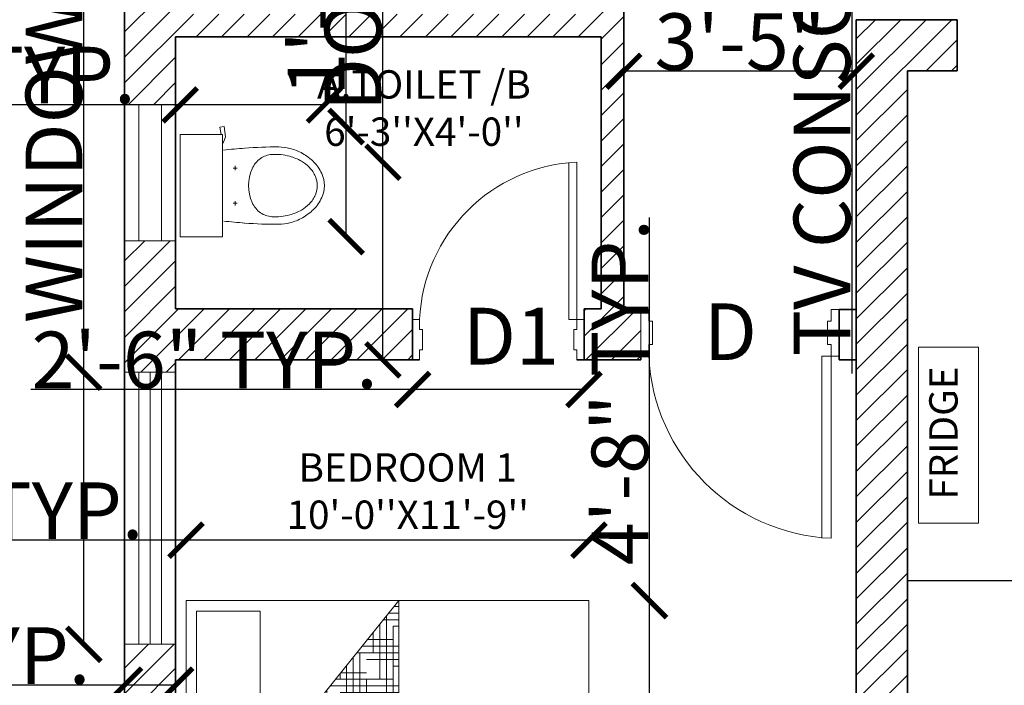
# Model space of a CAD drawing. Units: inches. Extents: x 1957 to 2456, y 1504 to 2088.
# Tile 3 of 6: x 2047 to 2220, y 1703 to 1820. Entities that reach past the tile are written whole.
import ezdxf

# ---------------------------------------------------------------- set-up
doc = ezdxf.new("R2010")
doc.units = ezdxf.units.IN
doc.header["$LTSCALE"] = 2
for name, color, linetype, lineweight in [('A-ANNO-DIMS', 2, 'Continuous', 18), ('A-ANNO-TEXT', 7, 'Continuous', 18), ('A-AREA-IDEN', 7, 'Continuous', 18), ('A-EQPM', 8, 'Continuous', 18), ('A-FLOR-FIXT', 8, 'Continuous', 18), ('A-FURN', 8, 'Continuous', 18), ('A-WALL-PATT', 8, 'Continuous', 13), ('Doors', 42, 'Continuous', 18), ('Kitchen', 60, 'Continuous', 25), ('Walls', 7, 'Continuous', 35), ('Windows', 140, 'Continuous', 18)]:
    doc.layers.add(name, color=color, linetype=linetype, lineweight=lineweight)
doc.styles.get("Standard").update_dxf_attribs({"font": 'arial.ttf'})
doc.dimstyles.get("Standard").update_dxf_attribs({"dimtxt": 10, "dimasz": 6, "dimexe": 0.18, "dimexo": 0.0625, "dimgap": 0.09, "dimtad": 1, "dimdec": 1, "dimzin": 0, "dimdsep": 46, "dimlunit": 4, "dimtxsty": 'Standard', "dimblk": 'ARCHTICK', "dimcen": 0.09, "dimse1": 1, "dimse2": 1, "dimadec": 0, "dimazin": 0, "dimtfac": 1, "dimtdec": 1, "dimtofl": 0, "dimtmove": 0, "dimatfit": 3, "dimfxl": 1, "dimtolj": 1, "dimtzin": 0, "dimarcsym": 0})

# ---------------------------------------------------------------- blocks, each defined once
blk = doc.blocks.new('*X4')
at = {"color": 0}
for p, q in [((20.25, 14.8125), (20.2772, 14.8125)), ((20.1875, 14.75), (20.1875, 14.7669)), ((20.199, 14.7812), (20.2772, 14.7812)), ((20.1487, 14.7188), (20.2772, 14.7188)), ((20.1562, 14.625), (20.1562, 14.7281)), ((20.1739, 14.75), (20.2772, 14.75)), ((20.25, 14.3194), (20.25, 14.75)), ((20.1236, 14.6875), (20.25, 14.6875)), ((20.125, 14.5), (20.125, 14.6893)), ((20.0938, 14.375), (20.0938, 14.6504)), ((20.0984, 14.6562), (20.125, 14.6562)), ((20.2188, 14.3091), (20.2188, 14.625)), ((20.25, 14.625), (20.2772, 14.625)), ((20.0625, 14.2573), (20.0625, 14.6116)), ((20.125, 14.5938), (20.2772, 14.5938)), ((19.9979, 14.5312), (20.2772, 14.5312)), ((20.023, 14.5625), (20.2772, 14.5625)), ((20.0312, 14.2469), (20.0312, 14.5727)), ((19.9727, 14.5), (20.25, 14.5)), ((20, 14.2366), (20, 14.5)), ((20.1875, 14.2987), (20.1875, 14.5)), ((19.9476, 14.4688), (20.125, 14.4688)), ((19.9062, 14.375), (19.9062, 14.4174)), ((19.9225, 14.4375), (20, 14.4375)), ((20.125, 14.4062), (20.2772, 14.4062)), ((20.25, 14.4375), (20.2772, 14.4375)), ((19.875, 14.25), (19.875, 14.3785)), ((19.9688, 14.2262), (19.9688, 14.375)), ((20, 14.375), (20.2772, 14.375)), ((20.1562, 14.2884), (20.1562, 14.375)), ((19.8125, 14.1744), (19.8125, 14.3008)), ((19.8219, 14.3125), (20.2291, 14.3125)), ((19.8438, 14.1848), (19.8438, 14.3397)), ((19.875, 14.3438), (20.2772, 14.3438)), ((19.7812, 14.1641), (19.7812, 14.262)), ((19.7967, 14.2812), (20.125, 14.2812)), ((19.7465, 14.2188), (19.875, 14.2188)), ((19.75, 14.1537), (19.75, 14.2231)), ((19.7716, 14.25), (20, 14.25)), ((19.9375, 14.2159), (19.9375, 14.25)), ((19.7213, 14.1875), (19.75, 14.1875)), ((19.7188, 14.0726), (19.7188, 14.1136)), ((19.7018, 14.0938), (19.7786, 14.0938)), ((19.75, 14.0338), (19.75, 14.1032)), ((19.7812, 13.9949), (19.7812, 14.0929)), ((19.8125, 14), (19.8125, 14.0825)), ((19.7269, 14.0625), (19.8728, 14.0625)), ((19.752, 14.0312), (19.875, 14.0312)), ((19.9062, 13.8396), (19.9062, 14.0514)), ((19.9375, 13.8007), (19.9375, 14.0411)), ((19.9688, 13.875), (19.9688, 14.0307)), ((19.875, 13.8784), (19.875, 14)), ((20, 14), (20, 14.0204)), ((20, 14), (20.0614, 14)), ((20.0625, 13.6454), (20.0625, 13.9996)), ((20.0938, 13.625), (20.0938, 13.9893)), ((20.125, 13.75), (20.125, 13.9789)), ((19.8275, 13.9375), (20.25, 13.9375)), ((19.875, 13.9688), (20.1557, 13.9688)), ((20.1562, 13.875), (20.1562, 13.9686)), ((20.25, 13.5), (20.25, 13.9375)), ((19.8526, 13.9062), (20.125, 13.9062)), ((19.8777, 13.875), (20, 13.875)), ((20.0312, 13.6842), (20.0312, 13.875)), ((20.125, 13.8438), (20.2772, 13.8438)), ((20.2188, 13.4511), (20.2188, 13.875)), ((20.25, 13.875), (20.2772, 13.875)), ((20, 13.8125), (20.2772, 13.8125)), ((19.9532, 13.7812), (20.2772, 13.7812)), ((19.9783, 13.75), (20.25, 13.75)), ((20, 13.723), (20, 13.75)), ((20.1875, 13.49), (20.1875, 13.75)), ((20.0035, 13.7188), (20.125, 13.7188)), ((20.125, 13.6562), (20.2772, 13.6562)), ((20.25, 13.6875), (20.2772, 13.6875)), ((20.0789, 13.625), (20.2772, 13.625)), ((20.1562, 13.5288), (20.1562, 13.625)), ((20.104, 13.5938), (20.2772, 13.5938)), ((20.1292, 13.5625), (20.25, 13.5625)), ((20.2046, 13.4688), (20.2772, 13.4688)), ((20.25, 13.5), (20.2772, 13.5)), ((20.2297, 13.4375), (20.2772, 13.4375)), ((20.2549, 13.4062), (20.2772, 13.4062))]:
    blk.add_line(p, q, dxfattribs=at)
blk = doc.blocks.new('MAT-P13')
for p, q in [((-0.75, 0), (0.75, 0)), ((-0.75, 0), (-0.75, -1.9)), ((0.75, 0), (0.75, -1.9)), ((-0.7, -0.05), (-0.7, -0.35)), ((-0.7, -0.05), (-0.05, -0.05)), ((-0.05, -0.35), (-0.05, -0.05)), ((0.05, -0.05), (0.7, -0.05)), ((0.05, -0.35), (0.05, -0.05)), ((0.7, -0.05), (0.7, -0.35)), ((-0.7, -0.35), (-0.05, -0.35)), ((0.05, -0.35), (0.7, -0.35)), ((-0.75, -1.0034), (0, -0.4)), ((0, -0.4), (-0.75, -1.0034)), ((0, -0.4), (-0.2, -1.0034)), ((0, -0.4), (0.2, -1.0034)), ((0, -0.4), (0.75, -1.0034)), ((-0.75, -1.0034), (-0.2, -1.0034)), ((0.2, -1.0034), (0.75, -1.0034)), ((0.75, -1.9), (-0.75, -1.9))]:
    blk.add_line(p, q)
at = {"xscale": -1, "rotation": 90}
blk.add_blockref('*X4', (14.1285, 19.2738), dxfattribs=at)
blk = doc.blocks.new('AP0B05')
for p, q in [((35, 100), (35, 880)), ((75, 100), (75, 878.9))]:
    blk.add_line(p, q)
for points in [[(0, 100), (0, -100), (35, -100), (35, -50), (50, -50), (50, 50), (35, 50), (35, 100)], [(850, 100), (850, -100), (815, -100), (815, -50), (800, -50), (800, 50), (815, 50), (815, 100)]]:
    blk.add_lwpolyline(points, close=True)
blk.add_lwpolyline([(35, 100), (75, 100)])
blk.add_arc((-2.4, 62.6), 818.3, 2.6212, 87.3788)
blk = doc.blocks.new('_ArchTick')
at = {"color": 0, "linetype": 'ByBlock', "const_width": 0.15}
blk.add_lwpolyline([(-0.5, -0.5), (0.5, 0.5)], dxfattribs=at)
blk = doc.blocks.new('*D10')
at = {"layer": 'A-ANNO-DIMS', "color": 0, "lineweight": -2, "transparency": 16777216}
blk.add_line((2194.03, 1811.13), (2153.03, 1811.13), dxfattribs=at)
at = {"layer": 'Defpoints', "color": 0, "transparency": 16777216}
for p in [(2153.03, 1820.22), (2194.03, 1820.22), (2153.03, 1811.13)]:
    blk.add_point(p, dxfattribs=at)
at = {"layer": 'A-ANNO-DIMS', "color": 0, "lineweight": -2, "transparency": 16777216, "xscale": 6, "yscale": 6, "zscale": 6, "rotation": 180}
blk.add_blockref('_ArchTick', (2153.03, 1811.13), dxfattribs=at)
at = {"layer": 'A-ANNO-DIMS', "color": 0, "lineweight": -2, "transparency": 16777216, "xscale": 6, "yscale": 6, "zscale": 6}
blk.add_blockref('_ArchTick', (2194.03, 1811.13), dxfattribs=at)
at = {"layer": 'A-ANNO-DIMS', "color": 0, "transparency": 16777216, "insert": (2173.53, 1816.33), "char_height": 10, "attachment_point": 5}
blk.add_mtext('\\A1;3\'-5"', dxfattribs=at)
blk = doc.blocks.new('toilet-1')
at = {"color": 0, "linetype": 'ByBlock'}
for p, q in [((-0.23, -0.02), (-0.23, -0.2116)), ((0.23, -0.02), (-0.23, -0.02)), ((0.23, -0.02), (0.23, -0.2116)), ((-0.23, -0.2116), (0.23, -0.2116)), ((0.1917, -0.2144), (0.2206, -0.225)), ((0.2206, -0.225), (0.266, -0.2187)), ((0.2633, -0.1997), (0.23, -0.2044)), ((0.266, -0.2187), (0.2633, -0.1997)), ((-0.0793, -0.2587), (-0.0793, -0.2778)), ((0.0794, -0.2587), (0.0794, -0.2778)), ((-0.0889, -0.2683), (-0.0697, -0.2683)), ((0.0889, -0.2683), (0.0698, -0.2683)), ((0, -0.6382), (0, -0.6382))]:
    blk.add_line(p, q, dxfattribs=at)
for centre, radius, start, end in [((3.5272, -0.6239), 3.7093, 173.6925, 175.1593), ((-3.527, -0.624), 3.7093, 4.8413, 6.3171), ((1.7368, -0.4519), 1.9109, 175.7698, 180.3758), ((-0.0312, -0.4465), 0.1114, 113.8997, 145.1485), ((0, -0.5169), 0.1884, 66.0939, 113.9061), ((0.0312, -0.4465), 0.1114, 34.8515, 66.1003), ((-1.7366, -0.4519), 1.9109, 359.6242, 4.2302), ((-0.0408, -0.4398), 0.0996, 145.1497, 175.881), ((0.0409, -0.4398), 0.0996, 4.119, 34.8503), ((0.0981, -0.4497), 0.2389, 175.8862, 195.5931), ((-0.098, -0.4497), 0.2389, 344.4069, 4.1138), ((0.0353, -0.463), 0.2093, 180.3747, 194.3375), ((-0.0351, -0.463), 0.2093, 345.6614, 359.6243), ((0.055, -0.458), 0.2297, 194.3353, 209.622), ((0.0961, -0.4503), 0.2369, 195.5969, 209.3771), ((-0.096, -0.4503), 0.2369, 330.6229, 344.4031), ((-0.0548, -0.458), 0.2297, 330.3788, 345.6655), ((0.0647, -0.4524), 0.2409, 209.6273, 224.5489), ((0.0232, -0.4913), 0.1532, 209.3871, 226.5438), ((-0.0231, -0.4913), 0.1532, 313.4562, 330.6129), ((-0.0645, -0.4524), 0.2409, 315.4504, 330.372), ((0.0152, -0.4997), 0.1416, 226.5501, 246.5527), ((-0.0151, -0.4997), 0.1416, 293.4473, 313.4499), ((0.0178, -0.4986), 0.1751, 224.552, 245.714), ((0.0004, -0.538), 0.132, 245.5845, 269.8782), ((0, -0.5347), 0.1034, 246.5493, 270.0042), ((0, -0.5347), 0.1034, 269.9958, 293.4507), ((-0.0002, -0.538), 0.132, 270.1216, 294.4153), ((-0.0176, -0.4986), 0.1751, 294.2865, 315.4485)]:
    blk.add_arc(centre, radius, start, end, dxfattribs=at)
blk = doc.blocks.new('WIN-48IN')
for p, q in [((0, 6.5), (48, 6.5)), ((0, 4.5), (48, 4.5)), ((0, 2.5), (48, 2.5))]:
    blk.add_line(p, q)
blk.add_lwpolyline([(0, 9), (48, 9), (48, 0), (0, 0)], close=True)
blk = doc.blocks.new('VENT-WIN-24IN')
for p, q in [((2.5, 0), (2.5, 24)), ((6.5, 0), (6.5, 24))]:
    blk.add_line(p, q)
blk.add_lwpolyline([(0, 0), (0, 24), (9, 24), (9, 0)], close=True)
blk = doc.blocks.new('*D21')
at = {"layer": 'A-ANNO-DIMS', "color": 0, "lineweight": -2, "transparency": 16777216}
for p, q in [((2110.57, 1795.08), (2110.57, 1937.02)), ((2110.57, 1760.22), (2110.57, 1795.08))]:
    blk.add_line(p, q, dxfattribs=at)
at = {"layer": 'Defpoints', "color": 0, "transparency": 16777216}
for p in [(2110.57, 1795.08), (2115.8, 1795.08), (2115.8, 1760.22)]:
    blk.add_point(p, dxfattribs=at)
at = {"layer": 'A-ANNO-DIMS', "color": 0, "lineweight": -2, "transparency": 16777216, "xscale": 6, "yscale": 6, "zscale": 6}
for p, rotation in [((2110.57, 1795.08), 90), ((2110.57, 1760.22), 270)]:
    blk.add_blockref('_ArchTick', p, dxfattribs=dict(at, rotation=rotation))
at = {"layer": 'A-ANNO-DIMS', "color": 0, "transparency": 16777216, "insert": (2105.3, 1869.05), "char_height": 10, "attachment_point": 5, "rotation": 90}
blk.add_mtext('\\A1;DOOR D1 2\'-11" TYP.', dxfattribs=at)
blk = doc.blocks.new('*D22')
at = {"layer": 'A-ANNO-DIMS', "color": 0, "lineweight": -2, "transparency": 16777216}
for p, q in [((2115.8, 1754.99), (2048.49, 1754.99)), ((2146.03, 1754.99), (2115.8, 1754.99))]:
    blk.add_line(p, q, dxfattribs=at)
at = {"layer": 'Defpoints', "color": 0, "transparency": 16777216}
for p in [(2115.8, 1760.22), (2146.03, 1760.22), (2115.8, 1754.99)]:
    blk.add_point(p, dxfattribs=at)
at = {"layer": 'A-ANNO-DIMS', "color": 0, "lineweight": -2, "transparency": 16777216, "xscale": 6, "yscale": 6, "zscale": 6, "rotation": 180}
blk.add_blockref('_ArchTick', (2115.8, 1754.99), dxfattribs=at)
at = {"layer": 'A-ANNO-DIMS', "color": 0, "lineweight": -2, "transparency": 16777216, "xscale": 6, "yscale": 6, "zscale": 6}
blk.add_blockref('_ArchTick', (2146.03, 1754.99), dxfattribs=at)
at = {"layer": 'A-ANNO-DIMS', "color": 0, "transparency": 16777216, "insert": (2079.14, 1760.19), "char_height": 10, "attachment_point": 5}
blk.add_mtext('\\A1;2\'-6" TYP.', dxfattribs=at)
blk = doc.blocks.new('*D23')
at = {"layer": 'A-ANNO-DIMS', "color": 0, "lineweight": -2, "transparency": 16777216}
for p, q in [((2057.83, 1758.05), (2057.83, 1890.77)), ((2057.83, 1710.05), (2057.83, 1758.05))]:
    blk.add_line(p, q, dxfattribs=at)
at = {"layer": 'Defpoints', "color": 0, "transparency": 16777216}
for p in [(2057.83, 1758.05), (2065.03, 1758.05), (2065.03, 1710.05)]:
    blk.add_point(p, dxfattribs=at)
at = {"layer": 'A-ANNO-DIMS', "color": 0, "lineweight": -2, "transparency": 16777216, "xscale": 6, "yscale": 6, "zscale": 6}
for p, rotation in [((2057.83, 1758.05), 90), ((2057.83, 1710.05), 270)]:
    blk.add_blockref('_ArchTick', p, dxfattribs=dict(at, rotation=rotation))
at = {"layer": 'A-ANNO-DIMS', "color": 0, "transparency": 16777216, "insert": (2052.57, 1827.41), "char_height": 10, "attachment_point": 5, "rotation": 90}
blk.add_mtext('\\A1;WINDOW 4\'-0" TYP.', dxfattribs=at)
blk = doc.blocks.new('*D24')
at = {"layer": 'A-ANNO-DIMS', "color": 0, "lineweight": -2, "transparency": 16777216}
for p, q in [((2065.03, 1702.85), (1997.9, 1702.85)), ((2074.03, 1702.85), (2065.03, 1702.85))]:
    blk.add_line(p, q, dxfattribs=at)
at = {"layer": 'Defpoints', "color": 0, "transparency": 16777216}
for p in [(2065.03, 1710.05), (2074.03, 1710.05), (2065.03, 1702.85)]:
    blk.add_point(p, dxfattribs=at)
at = {"layer": 'A-ANNO-DIMS', "color": 0, "lineweight": -2, "transparency": 16777216, "xscale": 6, "yscale": 6, "zscale": 6}
for p, rotation in [((2065.03, 1702.85), 179.9999999999986), ((2074.03, 1702.85), 359.9999999999986)]:
    blk.add_blockref('_ArchTick', p, dxfattribs=dict(at, rotation=rotation))
at = {"layer": 'A-ANNO-DIMS', "color": 0, "transparency": 16777216, "insert": (2028.47, 1708.05), "char_height": 10, "attachment_point": 5}
blk.add_mtext('\\A1;0\'-9" TYP.', dxfattribs=at)
blk = doc.blocks.new('*D28')
at = {"layer": 'A-ANNO-DIMS', "color": 0, "lineweight": -2, "transparency": 16777216}
for p, q in [((2065.03, 1829.62), (2074.03, 1829.62)), ((2074.03, 1829.62), (2141.17, 1829.62))]:
    blk.add_line(p, q, dxfattribs=at)
at = {"layer": 'Defpoints', "color": 0, "transparency": 16777216}
for p in [(2065.03, 1833.22), (2074.03, 1833.22), (2074.03, 1829.62)]:
    blk.add_point(p, dxfattribs=at)
at = {"layer": 'A-ANNO-DIMS', "color": 0, "lineweight": -2, "transparency": 16777216, "xscale": 6, "yscale": 6, "zscale": 6, "rotation": 180}
blk.add_blockref('_ArchTick', (2065.03, 1829.62), dxfattribs=at)
at = {"layer": 'A-ANNO-DIMS', "color": 0, "lineweight": -2, "transparency": 16777216, "xscale": 6, "yscale": 6, "zscale": 6}
blk.add_blockref('_ArchTick', (2074.03, 1829.62), dxfattribs=at)
at = {"layer": 'A-ANNO-DIMS', "color": 0, "transparency": 16777216, "insert": (2110.6, 1834.81), "char_height": 10, "attachment_point": 5}
blk.add_mtext('\\A1;0\'-9" TYP.', dxfattribs=at)
blk = doc.blocks.new('*D29')
at = {"layer": 'A-ANNO-DIMS', "color": 0, "lineweight": -2, "transparency": 16777216}
for p, q in [((2075.86, 1728.42), (1968.79, 1728.42)), ((2146.9, 1728.42), (2075.86, 1728.42))]:
    blk.add_line(p, q, dxfattribs=at)
at = {"layer": 'Defpoints', "color": 0, "transparency": 16777216}
for p in [(2075.86, 1728.42), (2075.86, 1717.76), (2146.9, 1717.76)]:
    blk.add_point(p, dxfattribs=at)
at = {"layer": 'A-ANNO-DIMS', "color": 0, "lineweight": -2, "transparency": 16777216, "xscale": 6, "yscale": 6, "zscale": 6, "rotation": 180}
blk.add_blockref('_ArchTick', (2075.86, 1728.42), dxfattribs=at)
at = {"layer": 'A-ANNO-DIMS', "color": 0, "lineweight": -2, "transparency": 16777216, "xscale": 6, "yscale": 6, "zscale": 6}
blk.add_blockref('_ArchTick', (2146.9, 1728.42), dxfattribs=at)
at = {"layer": 'A-ANNO-DIMS', "color": 0, "transparency": 16777216, "insert": (2019.32, 1733.61), "char_height": 10, "attachment_point": 5}
blk.add_mtext('\\A1;BED 5\'-11" TYP.', dxfattribs=at)
blk = doc.blocks.new('*D30')
at = {"layer": 'A-ANNO-DIMS', "color": 0, "lineweight": -2, "transparency": 16777216}
for p, q in [((2157.56, 1717.76), (2157.56, 1785.3)), ((2157.56, 1661.68), (2157.56, 1717.76))]:
    blk.add_line(p, q, dxfattribs=at)
at = {"layer": 'Defpoints', "color": 0, "transparency": 16777216}
for p in [(2146.9, 1717.76), (2157.56, 1717.76), (2146.9, 1661.68)]:
    blk.add_point(p, dxfattribs=at)
at = {"layer": 'A-ANNO-DIMS', "color": 0, "lineweight": -2, "transparency": 16777216, "xscale": 6, "yscale": 6, "zscale": 6}
for p, rotation in [((2157.56, 1717.76), 90), ((2157.56, 1661.68), 270)]:
    blk.add_blockref('_ArchTick', p, dxfattribs=dict(at, rotation=rotation))
at = {"layer": 'A-ANNO-DIMS', "color": 0, "transparency": 16777216, "insert": (2152.36, 1754.53), "char_height": 10, "attachment_point": 5, "rotation": 90}
blk.add_mtext('\\A1;4\'-8" TYP.', dxfattribs=at)
blk = doc.blocks.new('*D33')
at = {"layer": 'A-ANNO-DIMS', "color": 0, "lineweight": -2, "transparency": 16777216}
for p, q in [((2074.82, 1805.18), (1956.82, 1805.18)), ((2100.26, 1805.18), (2074.82, 1805.18))]:
    blk.add_line(p, q, dxfattribs=at)
at = {"layer": 'Defpoints', "color": 0, "transparency": 16777216}
for p in [(2074.82, 1805.18), (2074.82, 1801.36), (2100.26, 1801.36)]:
    blk.add_point(p, dxfattribs=at)
at = {"layer": 'A-ANNO-DIMS', "color": 0, "lineweight": -2, "transparency": 16777216, "xscale": 6, "yscale": 6, "zscale": 6, "rotation": 180}
blk.add_blockref('_ArchTick', (2074.82, 1805.18), dxfattribs=at)
at = {"layer": 'A-ANNO-DIMS', "color": 0, "lineweight": -2, "transparency": 16777216, "xscale": 6, "yscale": 6, "zscale": 6}
blk.add_blockref('_ArchTick', (2100.26, 1805.18), dxfattribs=at)
at = {"layer": 'A-ANNO-DIMS', "color": 0, "transparency": 16777216, "insert": (2012.82, 1810.44), "char_height": 10, "attachment_point": 5}
blk.add_mtext('\\A1;WC 2\'-1 1/2" TYP.', dxfattribs=at)
blk = doc.blocks.new('*D34')
at = {"layer": 'A-ANNO-DIMS', "color": 0, "lineweight": -2, "transparency": 16777216}
for p, q in [((2104.08, 1801.36), (2104.08, 1890.86)), ((2104.08, 1781.95), (2104.08, 1801.36))]:
    blk.add_line(p, q, dxfattribs=at)
at = {"layer": 'Defpoints', "color": 0, "transparency": 16777216}
for p in [(2100.26, 1801.36), (2104.08, 1801.36), (2100.26, 1781.95)]:
    blk.add_point(p, dxfattribs=at)
at = {"layer": 'A-ANNO-DIMS', "color": 0, "lineweight": -2, "transparency": 16777216, "xscale": 6, "yscale": 6, "zscale": 6}
for p, rotation in [((2104.08, 1801.36), 90), ((2104.08, 1781.95), 270)]:
    blk.add_blockref('_ArchTick', p, dxfattribs=dict(at, rotation=rotation))
at = {"layer": 'A-ANNO-DIMS', "color": 0, "transparency": 16777216, "insert": (2098.81, 1849.11), "char_height": 10, "attachment_point": 5, "rotation": 90}
blk.add_mtext('\\A1;1\'-7 1/2" TYP.', dxfattribs=at)
blk = doc.blocks.new('*D39')
at = {"layer": 'A-ANNO-DIMS', "color": 0, "lineweight": -2, "transparency": 16777216}
for p, q in [((2193.24, 1973.36), (2193.24, 1908.07)), ((2193.24, 1908.07), (2193.24, 1757.83))]:
    blk.add_line(p, q, dxfattribs=at)
at = {"layer": 'Defpoints', "color": 0, "transparency": 16777216}
for p in [(2203.03, 1973.36), (2193.24, 1908.07), (2203.03, 1908.07)]:
    blk.add_point(p, dxfattribs=at)
at = {"layer": 'A-ANNO-DIMS', "color": 0, "lineweight": -2, "transparency": 16777216, "xscale": 6, "yscale": 6, "zscale": 6}
for p, rotation in [((2193.24, 1973.36), 90), ((2193.24, 1908.07), 270)]:
    blk.add_blockref('_ArchTick', p, dxfattribs=dict(at, rotation=rotation))
at = {"layer": 'A-ANNO-DIMS', "color": 0, "transparency": 16777216, "insert": (2187.98, 1829.95), "char_height": 10, "attachment_point": 5, "rotation": 90}
blk.add_mtext('\\A1;TV CONSOLE 5\'-5 1/2"', dxfattribs=at)
blk = doc.blocks.new('*D52')
at = {"layer": 'A-ANNO-DIMS', "color": 0, "lineweight": -2, "transparency": 16777216}
blk.add_line((2040.63, 1610.22), (2040.63, 1710.05), dxfattribs=at)
at = {"layer": 'Defpoints', "color": 0, "transparency": 16777216}
for p in [(2040.63, 1710.05), (2074.03, 1710.05), (2074.03, 1610.22)]:
    blk.add_point(p, dxfattribs=at)
at = {"layer": 'A-ANNO-DIMS', "color": 0, "lineweight": -2, "transparency": 16777216, "xscale": 6, "yscale": 6, "zscale": 6}
for p, rotation in [((2040.63, 1710.05), 90), ((2040.63, 1610.22), 270)]:
    blk.add_blockref('_ArchTick', p, dxfattribs=dict(at, rotation=rotation))
at = {"layer": 'A-ANNO-DIMS', "color": 0, "transparency": 16777216, "insert": (2035.44, 1660.14), "char_height": 10, "attachment_point": 5, "rotation": 90}
blk.add_mtext('\\A1;8\'-4"', dxfattribs=at)
blk = doc.blocks.new('*D56')
at = {"layer": 'A-ANNO-DIMS', "color": 0, "lineweight": -2, "transparency": 16777216}
blk.add_line((2040.63, 1688.22), (2040.63, 1869.22), dxfattribs=at)
at = {"layer": 'Defpoints', "color": 0, "transparency": 16777216}
for p in [(2040.63, 1869.22), (2367.03, 1869.22), (2367.03, 1688.22)]:
    blk.add_point(p, dxfattribs=at)
at = {"layer": 'A-ANNO-DIMS', "color": 0, "lineweight": -2, "transparency": 16777216, "xscale": 6, "yscale": 6, "zscale": 6}
for p, rotation in [((2040.63, 1869.22), 90), ((2040.63, 1688.22), 270)]:
    blk.add_blockref('_ArchTick', p, dxfattribs=dict(at, rotation=rotation))
at = {"layer": 'A-ANNO-DIMS', "color": 0, "transparency": 16777216, "insert": (2035.44, 1778.72), "char_height": 10, "attachment_point": 5, "rotation": 90}
blk.add_mtext('\\A1;15\'-1"', dxfattribs=at)
blk = doc.blocks.new('*D57')
at = {"layer": 'A-ANNO-DIMS', "color": 0, "lineweight": -2, "transparency": 16777216}
for p, q in [((2040.63, 1781.22), (2040.63, 1813.04)), ((2040.63, 1769.22), (2040.63, 1781.22))]:
    blk.add_line(p, q, dxfattribs=at)
at = {"layer": 'Defpoints', "color": 0, "transparency": 16777216}
for p in [(2040.63, 1781.22), (2074.03, 1781.22), (2074.03, 1769.22)]:
    blk.add_point(p, dxfattribs=at)
at = {"layer": 'A-ANNO-DIMS', "color": 0, "lineweight": -2, "transparency": 16777216, "xscale": 6, "yscale": 6, "zscale": 6}
for p, rotation in [((2040.63, 1781.22), 90), ((2040.63, 1769.22), 270)]:
    blk.add_blockref('_ArchTick', p, dxfattribs=dict(at, rotation=rotation))
at = {"layer": 'A-ANNO-DIMS', "color": 0, "transparency": 16777216, "insert": (2035.44, 1800.13), "char_height": 10, "attachment_point": 5, "rotation": 90}
blk.add_mtext('\\A1;1\'-0"', dxfattribs=at)
blk = doc.blocks.new('*D58')
at = {"layer": 'A-ANNO-DIMS', "color": 0, "lineweight": -2, "transparency": 16777216}
for p, q in [((2040.63, 1833.22), (2040.63, 1865.04)), ((2040.63, 1821.22), (2040.63, 1833.22))]:
    blk.add_line(p, q, dxfattribs=at)
at = {"layer": 'Defpoints', "color": 0, "transparency": 16777216}
for p in [(2040.63, 1833.22), (2074.03, 1833.22), (2074.03, 1821.22)]:
    blk.add_point(p, dxfattribs=at)
at = {"layer": 'A-ANNO-DIMS', "color": 0, "lineweight": -2, "transparency": 16777216, "xscale": 6, "yscale": 6, "zscale": 6}
for p, rotation in [((2040.63, 1833.22), 90), ((2040.63, 1821.22), 270)]:
    blk.add_blockref('_ArchTick', p, dxfattribs=dict(at, rotation=rotation))
at = {"layer": 'A-ANNO-DIMS', "color": 0, "transparency": 16777216, "insert": (2035.44, 1852.13), "char_height": 10, "attachment_point": 5, "rotation": 90}
blk.add_mtext('\\A1;1\'-0"', dxfattribs=at)
blk = doc.blocks.new('*D59')
at = {"layer": 'A-ANNO-DIMS', "color": 0, "lineweight": -2, "transparency": 16777216}
blk.add_line((2074.03, 1513.82), (2115.8, 1513.82), dxfattribs=at)
at = {"layer": 'Defpoints', "color": 0, "transparency": 16777216}
for p in [(2074.03, 1760.22), (2115.8, 1760.22), (2115.8, 1513.82)]:
    blk.add_point(p, dxfattribs=at)
at = {"layer": 'A-ANNO-DIMS', "color": 0, "lineweight": -2, "transparency": 16777216, "xscale": 6, "yscale": 6, "zscale": 6, "rotation": 180}
blk.add_blockref('_ArchTick', (2074.03, 1513.82), dxfattribs=at)
at = {"layer": 'A-ANNO-DIMS', "color": 0, "lineweight": -2, "transparency": 16777216, "xscale": 6, "yscale": 6, "zscale": 6}
blk.add_blockref('_ArchTick', (2115.8, 1513.82), dxfattribs=at)
at = {"layer": 'A-ANNO-DIMS', "color": 0, "transparency": 16777216, "insert": (2094.91, 1519.02), "char_height": 10, "attachment_point": 5}
blk.add_mtext('\\A1;3\'-6"', dxfattribs=at)
blk = doc.blocks.new('*D62')
at = {"layer": 'A-ANNO-DIMS', "color": 0, "lineweight": -2, "transparency": 16777216}
for p, q in [((2074.03, 2045.62), (2108.63, 2045.62)), ((2108.63, 2045.62), (2172.63, 2045.62))]:
    blk.add_line(p, q, dxfattribs=at)
at = {"layer": 'Defpoints', "color": 0, "transparency": 16777216}
for p in [(2108.63, 2045.62), (2074.03, 1547.22), (2108.63, 1547.22)]:
    blk.add_point(p, dxfattribs=at)
at = {"layer": 'A-ANNO-DIMS', "color": 0, "lineweight": -2, "transparency": 16777216, "xscale": 6, "yscale": 6, "zscale": 6, "rotation": 180}
blk.add_blockref('_ArchTick', (2074.03, 2045.62), dxfattribs=at)
at = {"layer": 'A-ANNO-DIMS', "color": 0, "lineweight": -2, "transparency": 16777216, "xscale": 6, "yscale": 6, "zscale": 6}
blk.add_blockref('_ArchTick', (2108.63, 2045.62), dxfattribs=at)
at = {"layer": 'A-ANNO-DIMS', "color": 0, "transparency": 16777216, "insert": (2143.63, 2050.88), "char_height": 10, "attachment_point": 5}
blk.add_mtext('\\A1;2\'-10 1/2"', dxfattribs=at)
blk = doc.blocks.new('*D63')
at = {"layer": 'A-ANNO-DIMS', "color": 0, "lineweight": -2, "transparency": 16777216}
for p, q in [((2108.63, 2045.62), (2118.63, 2045.62)), ((2118.63, 2045.62), (2159.16, 2045.62))]:
    blk.add_line(p, q, dxfattribs=at)
at = {"layer": 'Defpoints', "color": 0, "transparency": 16777216}
for p in [(2118.63, 2045.62), (2108.63, 1547.22), (2118.63, 1547.22)]:
    blk.add_point(p, dxfattribs=at)
at = {"layer": 'A-ANNO-DIMS', "color": 0, "lineweight": -2, "transparency": 16777216, "xscale": 6, "yscale": 6, "zscale": 6, "rotation": 180}
blk.add_blockref('_ArchTick', (2108.63, 2045.62), dxfattribs=at)
at = {"layer": 'A-ANNO-DIMS', "color": 0, "lineweight": -2, "transparency": 16777216, "xscale": 6, "yscale": 6, "zscale": 6}
blk.add_blockref('_ArchTick', (2118.63, 2045.62), dxfattribs=at)
at = {"layer": 'A-ANNO-DIMS', "color": 0, "transparency": 16777216, "insert": (2141.89, 2050.81), "char_height": 10, "attachment_point": 5}
blk.add_mtext('\\A1;0\'-10"', dxfattribs=at)
blk = doc.blocks.new('*D67')
at = {"layer": 'A-ANNO-DIMS', "color": 0, "lineweight": -2, "transparency": 16777216}
for p, q in [((2040.63, 1761.57), (2040.63, 1817.8)), ((2040.63, 1735.04), (2040.63, 1761.57))]:
    blk.add_line(p, q, dxfattribs=at)
at = {"layer": 'Defpoints', "color": 0, "transparency": 16777216}
for p in [(2040.63, 1761.57), (2287.11, 1761.57), (2287.11, 1735.04)]:
    blk.add_point(p, dxfattribs=at)
at = {"layer": 'A-ANNO-DIMS', "color": 0, "lineweight": -2, "transparency": 16777216, "xscale": 6, "yscale": 6, "zscale": 6}
for p, rotation in [((2040.63, 1761.57), 90), ((2040.63, 1735.04), 270)]:
    blk.add_blockref('_ArchTick', p, dxfattribs=dict(at, rotation=rotation))
at = {"layer": 'A-ANNO-DIMS', "color": 0, "transparency": 16777216, "insert": (2035.37, 1792.69), "char_height": 10, "attachment_point": 5, "rotation": 90}
blk.add_mtext('\\A1;2\'-2 1/2"', dxfattribs=at)
blk = doc.blocks.new('*D68')
at = {"layer": 'A-ANNO-DIMS', "color": 0, "lineweight": -2, "transparency": 16777216}
for p, q in [((2395.43, 1821.22), (2395.43, 1853.98)), ((2395.43, 1817.22), (2395.43, 1821.22))]:
    blk.add_line(p, q, dxfattribs=at)
at = {"layer": 'Defpoints', "color": 0, "transparency": 16777216}
for p in [(2149.03, 1821.22), (2395.43, 1821.22), (2149.03, 1817.22)]:
    blk.add_point(p, dxfattribs=at)
at = {"layer": 'A-ANNO-DIMS', "color": 0, "lineweight": -2, "transparency": 16777216, "xscale": 6, "yscale": 6, "zscale": 6}
for p, rotation in [((2395.43, 1821.22), 90), ((2395.43, 1817.22), 270)]:
    blk.add_blockref('_ArchTick', p, dxfattribs=dict(at, rotation=rotation))
at = {"layer": 'A-ANNO-DIMS', "color": 0, "transparency": 16777216, "insert": (2390.24, 1840.6), "char_height": 10, "attachment_point": 5, "rotation": 90}
blk.add_mtext('\\A1;0\'-4"', dxfattribs=at)

msp = doc.modelspace()

# ---------------------------------------------------------------- hatches: boundary and pattern name
at = {"layer": 'A-WALL-PATT', "transparency": 33554585}
h = msp.add_hatch(dxfattribs=at)
h.set_pattern_fill('ANSI31', color=256)
h.paths.add_polyline_path([(2129.18, 2021.22), (2065.03, 2021.22), (2065.03, 1857.22), (2074.03, 1857.22), (2074.03, 1869.22), (2115.8, 1869.22), (2115.8, 1878.22), (2074.03, 1878.22), (2074.03, 2012.22), (2129.18, 2012.22)])
h.paths.add_polyline_path([(2209.75, 2021.22), (2189.18, 2021.22), (2189.18, 2012.22), (2194.03, 2012.22), (2194.03, 1878.22), (2190.56, 1878.22), (2190.56, 1869.22), (2203.03, 1869.22), (2203.03, 2012.22), (2209.75, 2012.22)])
h.paths.add_polyline_path([(2273.18, 2021.22), (2245.68, 2021.22), (2245.68, 2012.22), (2273.18, 2012.22)])
h.paths.add_polyline_path([(2371.03, 2021.22), (2333.18, 2021.22), (2333.18, 2012.22), (2362.03, 2012.22), (2362.03, 1968.25), (2371.03, 1968.25)])
h.paths.add_polyline_path([(2371.03, 1869.22), (2367.03, 1869.22), (2367.03, 1546.41), (2371.03, 1546.41)])
h.paths.add_polyline_path([(2317.03, 1820.22), (2247.38, 1820.22), (2247.38, 1811.22), (2308.03, 1811.22), (2308.03, 1697.22), (2284.03, 1697.22), (2284.03, 1688.22), (2317.03, 1688.22)])
h.paths.add_polyline_path([(2236.03, 1697.22), (2203.03, 1697.22), (2203.03, 1811.22), (2211.8, 1811.22), (2211.8, 1820.22), (2194.03, 1820.22), (2194.03, 1619.22), (2074.03, 1619.22), (2074.03, 1610.22), (2203.03, 1610.22), (2203.03, 1688.22), (2236.03, 1688.22)])
h.paths.add_polyline_path([(2153.03, 1869.22), (2155.49, 1869.22), (2155.49, 1877.47), (2155.49, 1878.22), (2146.03, 1878.22), (2146.03, 1871.1), (2146.03, 1869.22), (2149.03, 1869.22), (2149.03, 1821.22), (2074.03, 1821.22), (2074.03, 1833.22), (2065.03, 1833.22), (2065.03, 1805.22), (2074.03, 1805.22), (2074.03, 1817.22), (2149.03, 1817.22), (2149.03, 1769.22), (2146.03, 1769.22), (2146.03, 1760.22), (2153.03, 1760.22), (2156.02, 1760.22), (2156.02, 1760.87), (2156.02, 1769.11), (2153.03, 1769.11)])
h.paths.add_polyline_path([(2074.03, 1781.22), (2065.03, 1781.22), (2065.03, 1758.05), (2074.03, 1758.05), (2074.03, 1760.22), (2115.8, 1760.22), (2115.8, 1767.33), (2115.8, 1769.22), (2074.03, 1769.22)])
h = msp.add_hatch(dxfattribs=at)
h.set_pattern_fill('ANSI31', color=256)
h.paths.add_polyline_path([(2371.03, 1920.25), (2362.03, 1920.25), (2362.03, 1878.22), (2308.03, 1878.22), (2308.03, 1869.22), (2308.03, 1856.15), (2317.03, 1856.15), (2317.03, 1869.22), (2371.03, 1869.22)])
h.paths.add_polyline_path([(2074.03, 1710.05), (2065.03, 1710.05), (2065.03, 1538.22), (2203.03, 1538.22), (2220.79, 1538.22), (2220.79, 1547.22), (2203.03, 1547.22), (2074.03, 1547.22)])

# ---------------------------------------------------------------- linework, layer by layer
at = {"layer": 'A-EQPM'}
msp.add_lwpolyline([(2205.01, 1731.41), (2215.58, 1731.41), (2215.58, 1762.45), (2205.01, 1762.45)], close=True, dxfattribs=at)
at = {"layer": 'Kitchen'}
msp.add_line((2284.03, 1721.22), (2203.03, 1721.22), dxfattribs=at)
at = {"layer": 'Walls'}
for p, q in [((2065.03, 2021.22), (2065.03, 1538.22)), ((2153.03, 1869.22), (2153.03, 1769.11)), ((2194.03, 1820.22), (2194.03, 1619.22)), ((2211.8, 1820.22), (2194.03, 1820.22)), ((2211.8, 1820.22), (2211.8, 1811.22)), ((2149.03, 1817.22), (2074.03, 1817.22)), ((2074.03, 1817.22), (2074.03, 1769.22)), ((2149.03, 1817.22), (2149.03, 1769.22)), ((2203.03, 1811.22), (2203.03, 1697.22)), ((2211.8, 1811.22), (2203.03, 1811.22)), ((2115.8, 1769.22), (2074.03, 1769.22)), ((2115.8, 1760.22), (2115.8, 1769.22)), ((2149.03, 1769.22), (2146.03, 1769.22)), ((2146.03, 1769.22), (2146.03, 1760.22)), ((2156.02, 1769.11), (2153.03, 1769.11)), ((2191.03, 1760.22), (2191.03, 1769.11)), ((2191.03, 1769.11), (2194.03, 1769.11)), ((2074.03, 1760.22), (2074.03, 1547.22)), ((2117.04, 1760.22), (2074.03, 1760.22)), ((2153.03, 1760.22), (2144.79, 1760.22)), ((2156.02, 1760.22), (2153.03, 1760.22)), ((2156.02, 1760.87), (2156.02, 1760.22)), ((2194.03, 1760.22), (2191.03, 1760.22))]:
    msp.add_line(p, q, dxfattribs=at)

# ---------------------------------------------------------------- block references
at = {"layer": 'A-FLOR-FIXT', "xscale": 39.14169934857737, "yscale": 39.14169934857737, "zscale": 39.14169934857737, "rotation": 90}
msp.add_blockref('toilet-1', (2074.03, 1790.95), dxfattribs=at)
at = {"layer": 'A-FURN', "xscale": 37.39052698416379, "yscale": 37.39052698416379, "zscale": 37.39052698416379, "rotation": 90}
msp.add_blockref('MAT-P13', (2075.86, 1689.72), dxfattribs=at)
at = {"layer": 'Doors', "xscale": -0.035574224362456, "yscale": 0.035574224362456, "zscale": 0.035574224362456}
msp.add_blockref('AP0B05', (2146.03, 1763.78), dxfattribs=at)
at = {"layer": 'Doors', "xscale": 0.0411883758411932, "yscale": 0.0411883758411932, "zscale": 0.0411883758411932, "rotation": 180}
msp.add_blockref('AP0B05', (2191.03, 1764.99), dxfattribs=at)
at = {"layer": 'Windows'}
msp.add_blockref('VENT-WIN-24IN', (2065.03, 1781.22), dxfattribs=at)
at = {"layer": 'Windows', "rotation": 89.99999999999838}
msp.add_blockref('WIN-48IN', (2074.03, 1710.05), dxfattribs=at)

# ---------------------------------------------------------------- texts
at = {"layer": 'A-ANNO-TEXT'}
for s, p in [('D1', (2124.65, 1759.4)), ('D', (2167.13, 1760.18))]:
    msp.add_text(s, height=10, dxfattribs=at).set_placement(p)
at = {"layer": 'A-ANNO-TEXT', "insert": (2206.89, 1721.22), "char_height": 5, "attachment_point": 1, "rotation": 90}
msp.add_mtext_dynamic_manual_height_columns('\\pxqc;FRIDGE', width=52.1707, gutter_width=12.5, heights=[0], dxfattribs=at)
at = {"layer": 'A-AREA-IDEN', "char_height": 5, "attachment_point": 1}
for s, insert in [("\\pxqc;A.TOILET /B\\P6'-3''X4'-0''", (2091.72, 1811.3)), ("\\pxqc;BEDROOM 1\\P10'-0''X11'-9''", (2088.87, 1743.74))]:
    msp.add_mtext_dynamic_manual_height_columns(s, width=52.1707, gutter_width=12.5, heights=[0], dxfattribs=dict(at, insert=insert))

# ---------------------------------------------------------------- dimensions: what is measured, and where the dimension line sits
at = {"layer": 'A-ANNO-DIMS'}
for base, p1, p2, override, picture, middle in [((2108.63, 2045.62), (2074.03, 1547.22), (2108.63, 1547.22), {"dimdec": 1, "dimlfac": 1, "dimrnd": 0, "dimzin": 1, "dimdsep": 46, "dimlunit": 4, "dimfrac": 2}, '*D62', (2143.63, 2050.88)), ((2118.63, 2045.62), (2108.63, 1547.22), (2118.63, 1547.22), {"dimdec": 1, "dimlfac": 1, "dimrnd": 0, "dimzin": 1, "dimdsep": 46, "dimlunit": 4, "dimfrac": 2}, '*D63', (2141.89, 2050.81)), ((2153.03, 1811.13), (2194.03, 1820.22), (2153.03, 1820.22), {"dimclrd": 0, "dimclre": 0, "dimclrt": 0}, '*D10', (2173.53, 1816.33)), ((2115.8, 1513.82), (2074.03, 1760.22), (2115.8, 1760.22), {"dimdec": 1, "dimlfac": 1, "dimrnd": 0, "dimzin": 1, "dimdsep": 46, "dimlunit": 4, "dimfrac": 2}, '*D59', (2094.91, 1519.02))]:
    dim = msp.add_linear_dim(base=base, p1=p1, p2=p2, dimstyle='Standard', override=override, dxfattribs=at)
    dim.commit()
    dim.dimension.update_dxf_attribs({"geometry": picture, "text_midpoint": middle})
for base, p1, p2, angle, text, picture, middle in [((2193.24, 1908.07), (2203.03, 1973.36), (2203.03, 1908.07), 270, 'TV CONSOLE <>', '*D39', (2187.98, 1829.95)), ((2110.57, 1795.08), (2115.8, 1760.22), (2115.8, 1795.08), 90, 'DOOR D1 <> TYP.', '*D21', (2105.3, 1869.05)), ((2057.83, 1758.05), (2065.03, 1710.05), (2065.03, 1758.05), 90, 'WINDOW <> TYP.', '*D23', (2052.57, 1827.41)), ((2104.08, 1801.36), (2100.26, 1781.95), (2100.26, 1801.36), 90, '<> TYP.', '*D34', (2098.81, 1849.11)), ((2074.82, 1805.18), (2100.26, 1801.36), (2074.82, 1801.36), 180, 'WC <> TYP.', '*D33', (2012.82, 1810.44)), ((2157.56, 1717.76), (2146.9, 1661.68), (2146.9, 1717.76), 90, '<> TYP.', '*D30', (2152.36, 1754.53)), ((2115.8, 1754.99), (2146.03, 1760.22), (2115.8, 1760.22), 180, '<> TYP.', '*D22', (2079.14, 1760.19)), ((2075.86, 1728.42), (2146.9, 1717.76), (2075.86, 1717.76), 180, 'BED <> TYP.', '*D29', (2019.32, 1733.61)), ((2065.03, 1702.85), (2074.03, 1710.05), (2065.03, 1710.05), 180, '<> TYP.', '*D24', (2028.47, 1708.05))]:
    dim = msp.add_linear_dim(base=base, p1=p1, p2=p2, angle=angle, text=text, dimstyle='Standard', override={"dimdec": 1, "dimlfac": 1, "dimrnd": 0, "dimzin": 1, "dimdsep": 46, "dimlunit": 4, "dimfrac": 2}, dxfattribs=at)
    dim.commit()
    dim.dimension.update_dxf_attribs({"geometry": picture, "text_midpoint": middle})
for base, p1, p2, picture, middle in [((2040.63, 1869.22), (2367.03, 1688.22), (2367.03, 1869.22), '*D56', (2035.44, 1778.72)), ((2040.63, 1833.22), (2074.03, 1821.22), (2074.03, 1833.22), '*D58', (2035.44, 1852.13)), ((2395.43, 1821.22), (2149.03, 1817.22), (2149.03, 1821.22), '*D68', (2390.24, 1840.6)), ((2040.63, 1761.57), (2287.11, 1735.04), (2287.11, 1761.57), '*D67', (2035.37, 1792.69)), ((2040.63, 1781.22), (2074.03, 1769.22), (2074.03, 1781.22), '*D57', (2035.44, 1800.13)), ((2040.63, 1710.05), (2074.03, 1610.22), (2074.03, 1710.05), '*D52', (2035.44, 1660.14))]:
    dim = msp.add_linear_dim(base=base, p1=p1, p2=p2, angle=90, dimstyle='Standard', override={"dimdec": 1, "dimlfac": 1, "dimrnd": 0, "dimzin": 1, "dimdsep": 46, "dimlunit": 4, "dimfrac": 2}, dxfattribs=at)
    dim.commit()
    dim.dimension.update_dxf_attribs({"geometry": picture, "text_midpoint": middle})
dim = msp.add_linear_dim(base=(2074.03, 1829.62), p1=(2065.03, 1833.22), p2=(2074.03, 1833.22), text='<> TYP.', dimstyle='Standard', override={"dimdec": 1, "dimlfac": 1, "dimrnd": 0, "dimzin": 1, "dimdsep": 46, "dimlunit": 4, "dimfrac": 2}, dxfattribs=at)
dim.commit()
dim.dimension.update_dxf_attribs({"geometry": '*D28', "text_midpoint": (2110.6, 1834.81)})

doc.saveas('drawing.dxf')
